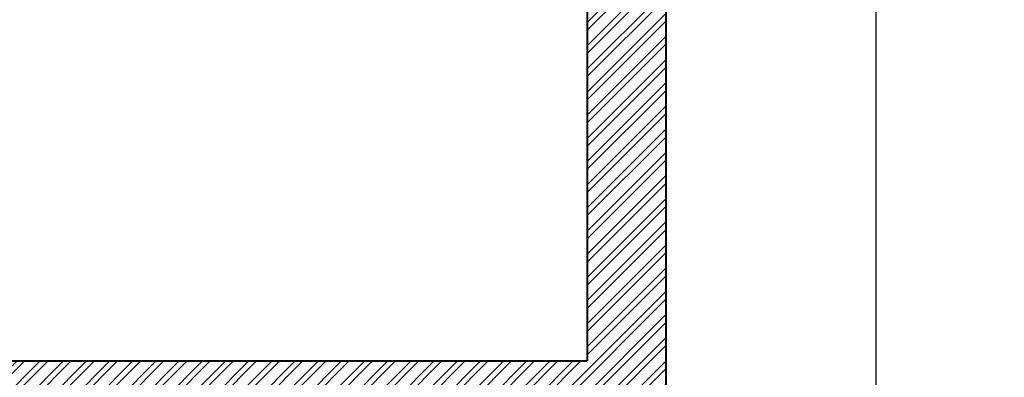
# Model space of a CAD drawing. Units: inches. Extents: x 528 to 2520, y -151 to 1354.
# Tile 10 of 41: x 812 to 924, y 1109 to 1150. Entities that reach past the tile are written whole.
import ezdxf

# ---------------------------------------------------------------- set-up
doc = ezdxf.new("R2010")
doc.units = ezdxf.units.IN
doc.header["$MEASUREMENT"] = 0
for name, color, linetype, lineweight in [('A-ANNO-DIMS', 2, 'Continuous', 18), ('A-WALL-PATT', 6, 'Continuous', 13), ('walls', 7, 'Continuous', 40)]:
    doc.layers.add(name, color=color, linetype=linetype, lineweight=lineweight)
doc.styles.get("Standard").update_dxf_attribs({"font": 'arial.ttf'})
doc.dimstyles.get("Standard").update_dxf_attribs({"dimtxt": 6, "dimasz": 2, "dimexe": 0.18, "dimexo": 0.0625, "dimgap": 0.09, "dimtad": 0, "dimtih": 1, "dimtoh": 1, "dimdec": 1, "dimzin": 0, "dimdsep": 46, "dimlunit": 3, "dimtxsty": 'Standard', "dimblk": 'ARCHTICK', "dimcen": 0.09, "dimadec": 0, "dimazin": 0, "dimtfac": 1, "dimtdec": 1, "dimtofl": 0, "dimtmove": 0, "dimatfit": 3, "dimfxl": 1, "dimtolj": 1, "dimtzin": 0, "dimarcsym": 0})

# ---------------------------------------------------------------- blocks, each defined once
blk = doc.blocks.new('_ArchTick')
at = {"color": 0, "linetype": 'ByBlock', "const_width": 0.15}
blk.add_lwpolyline([(-0.5, -0.5), (0.5, 0.5)], dxfattribs=at)
blk = doc.blocks.new('*D24')
at = {"layer": 'A-ANNO-DIMS', "color": 0, "lineweight": -2, "transparency": 16777216}
for p, q in [((885.76, 1317.1), (909.9, 1317.1)), ((909.72, 1317.1), (909.72, 1069.76)), ((909.72, 816.1), (909.72, 1063.45)), ((885.76, 816.1), (909.9, 816.1))]:
    blk.add_line(p, q, dxfattribs=at)
at = {"layer": 'Defpoints', "color": 0, "transparency": 16777216}
for p in [(885.7, 1317.1), (885.7, 816.1), (909.72, 816.1)]:
    blk.add_point(p, dxfattribs=at)
at = {"layer": 'A-ANNO-DIMS', "color": 0, "lineweight": -2, "transparency": 16777216, "xscale": 2, "yscale": 2, "zscale": 2}
for p, rotation in [((909.72, 1317.1), 90), ((909.72, 816.1), 270)]:
    blk.add_blockref('_ArchTick', p, dxfattribs=dict(at, rotation=rotation))
at = {"layer": 'A-ANNO-DIMS', "color": 0, "transparency": 16777216, "insert": (909.72, 1066.6), "char_height": 6, "attachment_point": 5}
blk.add_mtext('\\A1;41\'-9.0"', dxfattribs=at)

msp = doc.modelspace()

# ---------------------------------------------------------------- hatches: boundary and pattern name
at = {"layer": 'A-WALL-PATT'}
h = msp.add_hatch(dxfattribs=at)
h.set_pattern_fill('ANSI32', color=256, scale=5)
h.paths.add_polyline_path([(595.7, 1163.86), (586.7, 1163.86), (586.7, 969.1), (598.24, 969.1), (603.24, 969.1), (603.24, 974.1), (595.7, 974.1), (595.7, 1082.1), (691.7, 1082.1), (691.7, 1087.1), (691.7, 1106.1), (697.7, 1106.1), (697.7, 1111.1), (686.7, 1111.1), (686.7, 1087.1), (595.7, 1087.1)])
h.paths.add_polyline_path([(688.7, 974.1), (651.24, 974.1), (651.24, 969.1), (688.7, 969.1)])
h.paths.add_polyline_path([(885.7, 1171.37), (876.7, 1171.37), (876.7, 1111.1), (786.7, 1111.1), (786.7, 1106.1), (876.7, 1106.1), (876.7, 974.1), (786.7, 974.1), (786.7, 969.1), (876.7, 969.1), (876.7, 825.1), (834.7, 825.1), (834.7, 816.1), (885.7, 816.1)])
h.paths.add_polyline_path([(885.7, 1317.1), (876.65, 1317.1), (876.65, 1308.1), (876.7, 1308.1), (876.7, 1248.1), (822.7, 1248.1), (822.7, 1243.1), (876.7, 1243.1), (876.7, 1219.37), (885.7, 1219.37)])
h.paths.add_polyline_path([(852.65, 1317.1), (787.7, 1317.1), (787.7, 1248.1), (784.26, 1248.1), (784.26, 1243.1), (792.7, 1243.1), (792.7, 1249.1), (792.7, 1308.1), (852.65, 1308.1)])
h.paths.add_polyline_path([(684.7, 1317.1), (619.7, 1317.1), (619.7, 1308.1), (679.7, 1308.1), (679.7, 1248.1), (679.7, 1243.1), (684.7, 1243.1), (684.7, 1248.25)])
h.paths.add_polyline_path([(595.7, 1308.1), (595.7, 1317.1), (586.7, 1317.1), (586.7, 1211.86), (595.7, 1211.86), (595.7, 1243.1), (649.7, 1243.1), (649.7, 1248.1), (595.7, 1248.1)])
h.paths.add_polyline_path([(744.7, 969.1), (744.7, 974.1), (724.7, 974.1), (724.7, 969.1), (739.7, 969.1), (739.7, 874.29), (744.7, 874.29)])
h.paths.add_polyline_path([(739.7, 969.1), (727.7, 969.1), (727.7, 965.12), (730.74, 965.12), (730.74, 961.68), (734.43, 961.68), (734.43, 957.24), (739.7, 957.24)], flags=17)
h.paths.add_polyline_path([(786.7, 825.1), (744.7, 825.1), (744.7, 832.29), (739.7, 832.29), (739.7, 816.1), (786.7, 816.1)])

# ---------------------------------------------------------------- linework, layer by layer
at = {"layer": 'walls'}
for p, q in [((885.7, 1317.1), (885.7, 816.1)), ((876.7, 1243.1), (876.7, 1111.1)), ((786.7, 1111.1), (876.7, 1111.1))]:
    msp.add_line(p, q, dxfattribs=at)

# ---------------------------------------------------------------- dimensions: what is measured, and where the dimension line sits
at = {"layer": 'A-ANNO-DIMS'}
dim = msp.add_linear_dim(base=(909.72, 816.1), p1=(885.7, 1317.1), p2=(885.7, 816.1), angle=90, dimstyle='Standard', override={"dimclrd": 0, "dimclre": 0, "dimclrt": 0}, dxfattribs=at)
dim.commit()
dim.dimension.update_dxf_attribs({"geometry": '*D24', "text_midpoint": (909.72, 1066.6)})

doc.saveas('drawing.dxf')
